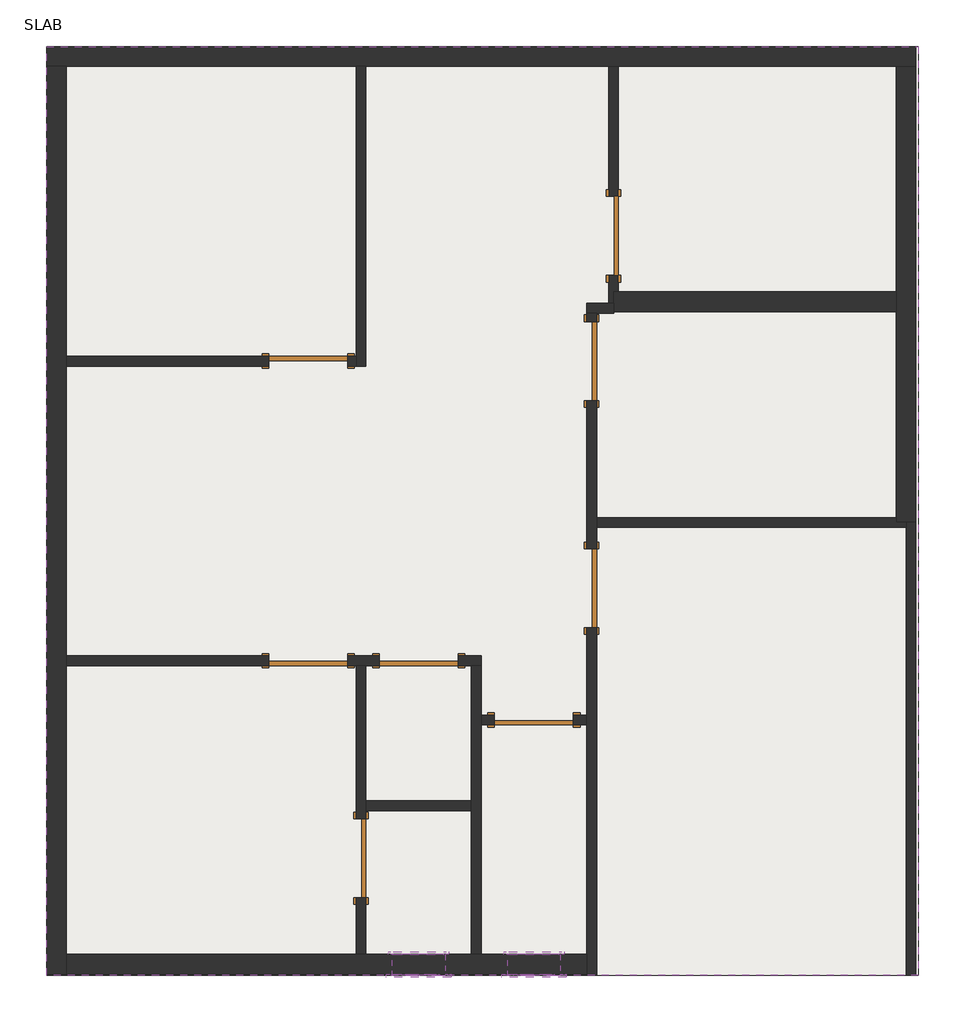
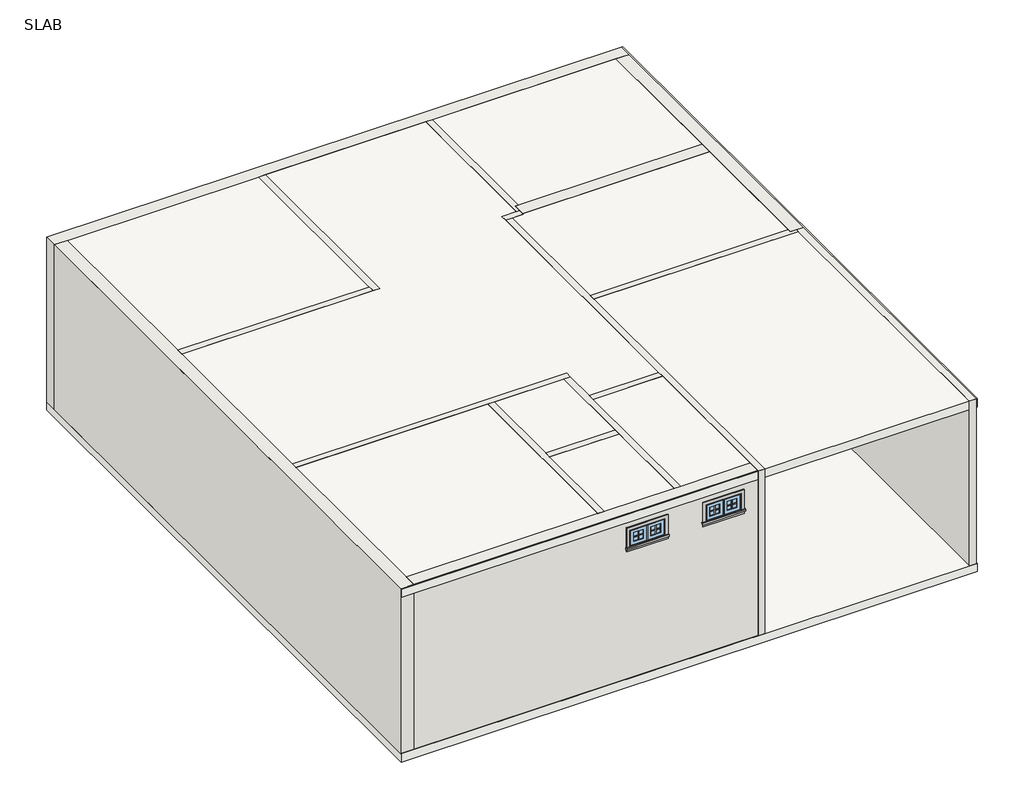
# One storey: 17 walls, 8 doors, 8 proxies, 2 slabs, 2 windows.
"""IFC4 building model written with IfcOpenShell, lengths in millimetres."""

from ifc_helpers import new_model, si_unit, frame, origin, place, context, project, spatial, polyline, outline, extrude, faceted_brep, transform, mapped, element, save
from components import muntin_pattern_2x2_muntin_pattern_2x2_4939cdd6, muntin_pattern_2x2_muntin_pattern_2x2_7edc5815, trim_window_exterior_flat_with_sill_281d40e2, trim_window_interior_flat_picture_frame_d1e4ee8f, door_305aa2a5, door_e5f9f3c4, window_375d1de9

model = new_model("IFC4")

# Units and contexts
model_context = context("Model", 3, world=origin())
ifc_project = project(units=[si_unit("LENGTHUNIT", "METRE", prefix="MILLI")], contexts=[model_context])

# Site, building, storey
site = spatial("IfcSite", under=ifc_project)
building = spatial("IfcBuilding", under=site)
storey = spatial("IfcBuildingStorey", under=building, Name="SLAB", Elevation=3657.6)

# Proxies
placement = place(None, origin())
muntin_pattern_2x2_muntin_pattern_2x2_shape = muntin_pattern_2x2_muntin_pattern_2x2_4939cdd6(model_context)
element("IfcBuildingElementProxy", 1, Name="Muntin Pattern_2x2 : Muntin Pattern_2x2", ObjectType="Muntin Pattern_2x2 : Muntin Pattern_2x2", at=placement, inside=storey, context=model_context, shape_type="MappedRepresentation", body=[
    mapped(muntin_pattern_2x2_muntin_pattern_2x2_shape, transform((-5153.2054063, 91.6138401, 6165.85), x_axis=(-1.0, 0.0, 0.0), y_axis=(0.0, -1.0, 0.0), z_axis=(0.0, 0.0, 1.0))),
])
element("IfcBuildingElementProxy", 2, Name="Muntin Pattern_2x2 : Muntin Pattern_2x2", ObjectType="Muntin Pattern_2x2 : Muntin Pattern_2x2", at=placement, inside=storey, context=model_context, shape_type="MappedRepresentation", body=[
    mapped(muntin_pattern_2x2_muntin_pattern_2x2_shape, transform((-3819.7054063, 91.6138401, 6165.85), x_axis=(-1.0, 0.0, 0.0), y_axis=(0.0, -1.0, 0.0), z_axis=(0.0, 0.0, 1.0))),
])
muntin_pattern_2x2_muntin_pattern_2x2_2_shape = muntin_pattern_2x2_muntin_pattern_2x2_7edc5815(model_context)
element("IfcBuildingElementProxy", 3, Name="Muntin Pattern_2x2 : Muntin Pattern_2x2", ObjectType="Muntin Pattern_2x2 : Muntin Pattern_2x2", at=placement, inside=storey, context=model_context, shape_type="MappedRepresentation", body=[
    mapped(muntin_pattern_2x2_muntin_pattern_2x2_2_shape, transform((-5454.8304063, 91.6138401, 6165.85), x_axis=(1.0, 0.0, 0.0), y_axis=(0.0, 1.0, 0.0), z_axis=(0.0, 0.0, 1.0))),
])
element("IfcBuildingElementProxy", 4, Name="Muntin Pattern_2x2 : Muntin Pattern_2x2", ObjectType="Muntin Pattern_2x2 : Muntin Pattern_2x2", at=placement, inside=storey, context=model_context, shape_type="MappedRepresentation", body=[
    mapped(muntin_pattern_2x2_muntin_pattern_2x2_2_shape, transform((-4121.3304063, 91.6138401, 6165.85), x_axis=(1.0, 0.0, 0.0), y_axis=(0.0, 1.0, 0.0), z_axis=(0.0, 0.0, 1.0))),
])
trim_window_exterior_flat_with_sill_shape = trim_window_exterior_flat_with_sill_281d40e2(model_context)
element("IfcBuildingElementProxy", 5, Name="Trim-Window-Exterior-Flat : with Sill", ObjectType="Trim-Window-Exterior-Flat : with Sill", at=placement, inside=storey, context=model_context, shape_type="MappedRepresentation", body=[
    mapped(trim_window_exterior_flat_with_sill_shape, transform((-5304.0179063, 82.0888401, 6400.8), x_axis=(1.0, 0.0, 0.0), y_axis=(0.0, 0.0, 1.0), z_axis=(0.0, -1.0, 0.0))),
])
element("IfcBuildingElementProxy", 6, Name="Trim-Window-Exterior-Flat : with Sill", ObjectType="Trim-Window-Exterior-Flat : with Sill", at=placement, inside=storey, context=model_context, shape_type="MappedRepresentation", body=[
    mapped(trim_window_exterior_flat_with_sill_shape, transform((-3970.5179063, 82.0888401, 6400.8), x_axis=(1.0, 0.0, 0.0), y_axis=(0.0, 0.0, 1.0), z_axis=(0.0, -1.0, 0.0))),
])
trim_window_interior_flat_picture_frame_shape = trim_window_interior_flat_picture_frame_d1e4ee8f(model_context)
element("IfcBuildingElementProxy", 7, Name="Trim-Window-Interior-Flat : Picture Frame", ObjectType="Trim-Window-Interior-Flat : Picture Frame", at=placement, inside=storey, context=model_context, shape_type="MappedRepresentation", body=[
    mapped(trim_window_interior_flat_picture_frame_shape, transform((-5304.0179063, 310.6888401, 6400.8), x_axis=(-1.0, 0.0, 0.0), y_axis=(0.0, 0.0, 1.0), z_axis=(0.0, 1.0, 0.0))),
])
element("IfcBuildingElementProxy", 8, Name="Trim-Window-Interior-Flat : Picture Frame", ObjectType="Trim-Window-Interior-Flat : Picture Frame", at=placement, inside=storey, context=model_context, shape_type="MappedRepresentation", body=[
    mapped(trim_window_interior_flat_picture_frame_shape, transform((-3970.5179063, 310.6888401, 6400.8), x_axis=(-1.0, 0.0, 0.0), y_axis=(0.0, 0.0, 1.0), z_axis=(0.0, 1.0, 0.0))),
])

# Doors
door_shape = door_305aa2a5(model_context)
element("IfcDoor", 9, ObjectType="Single-Flush : 36\" x 84\"", at=placement, inside=storey, context=model_context, shape_type="MappedRepresentation", body=[
    mapped(door_shape, transform((-5970.7679063, 1421.9388401, 3657.6), x_axis=(0.0, 1.0, 0.0), y_axis=(-1.0, 0.0, 0.0), z_axis=(0.0, 0.0, 1.0))),
])
element("IfcDoor", 10, ObjectType="Single-Flush : 36\" x 84\"", at=placement, inside=storey, context=model_context, shape_type="MappedRepresentation", body=[
    mapped(door_shape, transform((-5304.0179063, 3707.9388401, 3657.6), x_axis=(1.0, 0.0, 0.0), y_axis=(0.0, 1.0, 0.0), z_axis=(0.0, 0.0, 1.0))),
])
element("IfcDoor", 11, ObjectType="Single-Flush : 36\" x 84\"", at=placement, inside=storey, context=model_context, shape_type="MappedRepresentation", body=[
    mapped(door_shape, transform((-6580.3679063, 3707.9388401, 3657.6), x_axis=(1.0, 0.0, 0.0), y_axis=(0.0, 1.0, 0.0), z_axis=(0.0, 0.0, 1.0))),
])
element("IfcDoor", 12, ObjectType="Single-Flush : 36\" x 84\"", at=placement, inside=storey, context=model_context, shape_type="MappedRepresentation", body=[
    mapped(door_shape, transform((-3303.7679063, 7175.0388401, 3657.6), x_axis=(0.0, 1.0, 0.0), y_axis=(-1.0, 0.0, 0.0), z_axis=(0.0, 0.0, 1.0))),
])
door_2_shape = door_e5f9f3c4(model_context)
element("IfcDoor", 13, ObjectType="Single-Flush : 36\" x 84\"", at=placement, inside=storey, context=model_context, shape_type="MappedRepresentation", body=[
    mapped(door_2_shape, transform((-3303.7679063, 4546.1388401, 3657.6), x_axis=(0.0, -1.0, 0.0), y_axis=(1.0, 0.0, 0.0), z_axis=(0.0, 0.0, 1.0))),
])
element("IfcDoor", 14, ObjectType="Single-Flush : 36\" x 84\"", at=placement, inside=storey, context=model_context, shape_type="MappedRepresentation", body=[
    mapped(door_2_shape, transform((-3970.5179063, 3022.1388401, 3657.6), x_axis=(-1.0, 0.0, 0.0), y_axis=(0.0, -1.0, 0.0), z_axis=(0.0, 0.0, 1.0))),
])
element("IfcDoor", 15, ObjectType="Single-Flush : 36\" x 84\"", at=placement, inside=storey, context=model_context, shape_type="MappedRepresentation", body=[
    mapped(door_2_shape, transform((-6580.3679063, 7175.0388401, 3657.6), x_axis=(1.0, 0.0, 0.0), y_axis=(0.0, 1.0, 0.0), z_axis=(0.0, 0.0, 1.0))),
])
element("IfcDoor", 16, ObjectType="Single-Flush : 36\" x 84\"", at=placement, inside=storey, context=model_context, shape_type="MappedRepresentation", body=[
    mapped(door_2_shape, transform((-3049.7679063, 8622.8388401, 3657.6), x_axis=(0.0, -1.0, 0.0), y_axis=(1.0, 0.0, 0.0), z_axis=(0.0, 0.0, 1.0))),
])

# Slabs
element("IfcSlab", 17, ObjectType="SLAB 6\"", at=placement, inside=storey, context=model_context, shape_type="SweptSolid", body=[
    extrude(outline(polyline([(449.0820937, 10813.5888401), (474.4820937, 10813.5888401), (474.4820937, 69.3888401), (-9609.3179063, 69.3888401), (-9609.3179063, 10813.5888401), (449.0820937, 10813.5888401)])), frame((0.0, 0.0, 3505.2), z_axis=(0.0, 0.0, 1.0), x_axis=(1.0, 0.0, 0.0)), (0.0, 0.0, 1.0), 152.4),
])
element("IfcSlab", 18, ObjectType="SLAB 6\"", at=placement, inside=storey, context=model_context, shape_type="SweptSolid", body=[
    extrude(outline(polyline([(449.0820937, 10813.5888401), (474.4820937, 10813.5888401), (474.4820937, 69.3888401), (-9609.3179063, 69.3888401), (-9609.3179063, 10813.5888401), (449.0820937, 10813.5888401)])), frame((0.0, 0.0, 6553.2), z_axis=(0.0, 0.0, 1.0), x_axis=(1.0, 0.0, 0.0)), (0.0, 0.0, 1.0), 152.4),
])

# Walls
element("IfcWall", 19, ObjectType="wall 4.5\"", at=placement, inside=storey, context=model_context, shape_type="Brep", body=[
    faceted_brep([(-3246.6179063, 7632.2388401, 5791.2), (-3246.6179063, 7632.2388401, 3657.6), (-3246.6179063, 7727.4888401, 3657.6), (-3246.6179063, 7727.4888401, 6705.6), (-3246.6179063, 5365.2888401, 6705.6), (-3246.6179063, 5250.9888401, 6705.6), (-3246.6179063, 69.3888401, 6705.6), (-3246.6179063, 69.3888401, 3657.6), (-3246.6179063, 4088.9388401, 3657.6), (-3246.6179063, 4088.9388401, 5791.2), (-3246.6179063, 5003.3388401, 5791.2), (-3246.6179063, 5003.3388401, 3657.6), (-3246.6179063, 5250.9888401, 3657.6), (-3246.6179063, 5365.2888401, 3657.6), (-3246.6179063, 6717.8388401, 3657.6), (-3246.6179063, 6717.8388401, 5791.2), (-3360.9179063, 7727.4888401, 3657.6), (-3360.9179063, 7632.2388401, 3657.6), (-3360.9179063, 7632.2388401, 5791.2), (-3360.9179063, 6717.8388401, 5791.2), (-3360.9179063, 6717.8388401, 3657.6), (-3360.9179063, 5003.3388401, 3657.6), (-3360.9179063, 5003.3388401, 5791.2), (-3360.9179063, 4088.9388401, 5791.2), (-3360.9179063, 4088.9388401, 3657.6), (-3360.9179063, 3079.2888401, 3657.6), (-3360.9179063, 2964.9888401, 3657.6), (-3360.9179063, 69.3888401, 3657.6), (-3360.9179063, 69.3888401, 6705.6), (-3360.9179063, 2964.9888401, 6705.6), (-3360.9179063, 3079.2888401, 6705.6), (-3360.9179063, 7727.4888401, 6705.6)], [[[0, 1, 2, 3, 4, 5, 6, 7, 8, 9, 10, 11, 12, 13, 14, 15]], [[16, 17, 18, 19, 20, 21, 22, 23, 24, 25, 26, 27, 28, 29, 30, 31]], [[27, 26, 25, 24, 8, 7]], [[2, 1, 17, 16]], [[14, 13, 12, 11, 21, 20]], [[6, 5, 4, 3, 31, 30, 29, 28]], [[7, 6, 28, 27]], [[3, 2, 16, 31]], [[9, 8, 24, 23]], [[10, 9, 23, 22]], [[11, 10, 22, 21]], [[18, 17, 1, 0]], [[19, 18, 0, 15]], [[20, 19, 15, 14]]]),
])
element("IfcWall", 20, ObjectType="wall 4.5\"", at=placement, inside=storey, context=model_context, shape_type="Brep", body=[
    faceted_brep([(334.7820937, 5308.1388401, 3657.6), (334.7820937, 5250.9888401, 3657.6), (334.7820937, 69.3888401, 3657.6), (334.7820937, 69.3888401, 6705.6), (334.7820937, 5250.9888401, 6705.6), (334.7820937, 5308.1388401, 6705.6), (449.0820937, 5308.1388401, 3657.6), (449.0820937, 5308.1388401, 6705.6), (449.0820937, 69.3888401, 6705.6), (449.0820937, 69.3888401, 3657.6)], [[[0, 1, 2, 3, 4, 5]], [[6, 7, 8, 9]], [[2, 1, 0, 6, 9]], [[3, 2, 9, 8]], [[5, 4, 3, 8, 7]], [[0, 5, 7, 6]]]),
])
element("IfcWall", 21, ObjectType="wall 4.5\"", at=placement, inside=storey, context=model_context, shape_type="SweptSolid", body=[
    extrude(outline(polyline([(334.7820937, 5250.9888401), (-3246.6179063, 5250.9888401), (-3246.6179063, 5365.2888401), (220.4820937, 5365.2888401), (220.4820937, 5308.1388401), (334.7820937, 5308.1388401), (334.7820937, 5250.9888401)])), frame((0.0, 0.0, 3657.6), z_axis=(0.0, 0.0, 1.0), x_axis=(1.0, 0.0, 0.0)), (0.0, 0.0, 1.0), 3048.0),
])
element("IfcWall", 22, ObjectType="wall 4.5\"", at=placement, inside=storey, context=model_context, shape_type="Brep", body=[
    faceted_brep([(-3106.9179063, 8165.6388401, 5791.2), (-3106.9179063, 8165.6388401, 3657.6), (-3106.9179063, 7841.7888401, 3657.6), (-3106.9179063, 7841.7888401, 6705.6), (-3106.9179063, 10584.9888401, 6705.6), (-3106.9179063, 10584.9888401, 3657.6), (-3106.9179063, 9080.0388401, 3657.6), (-3106.9179063, 9080.0388401, 5791.2), (-2992.6179063, 7975.1388401, 3657.6), (-2992.6179063, 8165.6388401, 3657.6), (-2992.6179063, 8165.6388401, 5791.2), (-2992.6179063, 9080.0388401, 5791.2), (-2992.6179063, 9080.0388401, 3657.6), (-2992.6179063, 10584.9888401, 3657.6), (-2992.6179063, 10584.9888401, 6705.6), (-2992.6179063, 7975.1388401, 6705.6), (-3049.7679063, 7975.1388401, 3657.6), (-3049.7679063, 7841.7888401, 3657.6), (-3049.7679063, 7841.7888401, 6705.6), (-3049.7679063, 7975.1388401, 6705.6)], [[[0, 1, 2, 3, 4, 5, 6, 7]], [[8, 9, 10, 11, 12, 13, 14, 15]], [[6, 5, 13, 12]], [[2, 1, 9, 8, 16, 17]], [[4, 3, 18, 19, 15, 14]], [[5, 4, 14, 13]], [[3, 2, 17, 18]], [[17, 16, 19, 18]], [[16, 8, 15, 19]], [[10, 9, 1, 0]], [[11, 10, 0, 7]], [[12, 11, 7, 6]]]),
])
element("IfcWall", 23, ObjectType="wall 4.5\"", at=placement, inside=storey, context=model_context, shape_type="Brep", body=[
    faceted_brep([(-6027.9179063, 10584.9888401, 3657.6), (-6027.9179063, 7232.1888401, 3657.6), (-6027.9179063, 7117.8888401, 3657.6), (-6027.9179063, 7117.8888401, 6705.6), (-6027.9179063, 7232.1888401, 6705.6), (-6027.9179063, 10584.9888401, 6705.6), (-5913.6179063, 10584.9888401, 3657.6), (-5913.6179063, 10584.9888401, 6705.6), (-5913.6179063, 7117.8888401, 6705.6), (-5913.6179063, 7117.8888401, 3657.6)], [[[0, 1, 2, 3, 4, 5]], [[6, 7, 8, 9]], [[2, 1, 0, 6, 9]], [[5, 4, 3, 8, 7]], [[0, 5, 7, 6]], [[3, 2, 9, 8]]]),
])
element("IfcWall", 24, ObjectType="wall 4.5\"", at=placement, inside=storey, context=model_context, shape_type="SweptSolid", body=[
    extrude(outline(polyline([(5791.2, -6123.1679063), (3657.6, -6123.1679063), (3657.6, -6027.9179063), (6705.6, -6027.9179063), (6705.6, -9380.7179063), (3657.6, -9380.7179063), (3657.6, -7037.5679063), (5791.2, -7037.5679063), (5791.2, -6123.1679063)])), frame((0.0, 7117.8888401, 0.0), z_axis=(0.0, 1.0, 0.0), x_axis=(0.0, 0.0, 1.0)), (0.0, 0.0, 1.0), 114.3),
])
element("IfcWall", 25, ObjectType="wall 4.5\"", at=placement, inside=storey, context=model_context, shape_type="Brep", body=[
    faceted_brep([(-6123.1679063, 3650.7888401, 5791.2), (-6123.1679063, 3650.7888401, 3657.6), (-6027.9179063, 3650.7888401, 3657.6), (-5913.6179063, 3650.7888401, 3657.6), (-5761.2179063, 3650.7888401, 3657.6), (-5761.2179063, 3650.7888401, 5791.2), (-4846.8179063, 3650.7888401, 5791.2), (-4846.8179063, 3650.7888401, 3657.6), (-4694.4179063, 3650.7888401, 3657.6), (-4580.1179063, 3650.7888401, 3657.6), (-4580.1179063, 3650.7888401, 6705.6), (-4694.4179063, 3650.7888401, 6705.6), (-5913.6179063, 3650.7888401, 6705.6), (-6027.9179063, 3650.7888401, 6705.6), (-9380.7179063, 3650.7888401, 6705.6), (-9380.7179063, 3650.7888401, 3657.6), (-7037.5679063, 3650.7888401, 3657.6), (-7037.5679063, 3650.7888401, 5791.2), (-5761.2179063, 3765.0888401, 3657.6), (-6123.1679063, 3765.0888401, 3657.6), (-6123.1679063, 3765.0888401, 5791.2), (-7037.5679063, 3765.0888401, 5791.2), (-7037.5679063, 3765.0888401, 3657.6), (-9380.7179063, 3765.0888401, 3657.6), (-9380.7179063, 3765.0888401, 6705.6), (-4580.1179063, 3765.0888401, 6705.6), (-4580.1179063, 3765.0888401, 3657.6), (-4846.8179063, 3765.0888401, 3657.6), (-4846.8179063, 3765.0888401, 5791.2), (-5761.2179063, 3765.0888401, 5791.2)], [[[0, 1, 2, 3, 4, 5, 6, 7, 8, 9, 10, 11, 12, 13, 14, 15, 16, 17]], [[18, 19, 20, 21, 22, 23, 24, 25, 26, 27, 28, 29]], [[9, 8, 7, 27, 26]], [[16, 15, 23, 22]], [[4, 3, 2, 1, 19, 18]], [[14, 13, 12, 11, 10, 25, 24]], [[15, 14, 24, 23]], [[10, 9, 26, 25]], [[28, 27, 7, 6]], [[29, 28, 6, 5]], [[18, 29, 5, 4]], [[20, 19, 1, 0]], [[21, 20, 0, 17]], [[22, 21, 17, 16]]]),
])
element("IfcWall", 26, ObjectType="wall 4.5\"", at=placement, inside=storey, context=model_context, shape_type="Brep", body=[
    faceted_brep([(-4694.4179063, 3650.7888401, 3657.6), (-4694.4179063, 2088.6888401, 3657.6), (-4694.4179063, 1974.3888401, 3657.6), (-4694.4179063, 310.6888401, 3657.6), (-4694.4179063, 310.6888401, 6705.6), (-4694.4179063, 1974.3888401, 6705.6), (-4694.4179063, 2088.6888401, 6705.6), (-4694.4179063, 3650.7888401, 6705.6), (-4580.1179063, 3650.7888401, 3657.6), (-4580.1179063, 3650.7888401, 6705.6), (-4580.1179063, 3079.2888401, 6705.6), (-4580.1179063, 2964.9888401, 6705.6), (-4580.1179063, 310.6888401, 6705.6), (-4580.1179063, 310.6888401, 3657.6), (-4580.1179063, 2964.9888401, 3657.6), (-4580.1179063, 3079.2888401, 3657.6)], [[[0, 1, 2, 3, 4, 5, 6, 7]], [[8, 9, 10, 11, 12, 13, 14, 15]], [[3, 2, 1, 0, 8, 15, 14, 13]], [[7, 6, 5, 4, 12, 11, 10, 9]], [[0, 7, 9, 8]], [[4, 3, 13, 12]]]),
])
element("IfcWall", 27, ObjectType="wall 4.5\"", at=placement, inside=storey, context=model_context, shape_type="Brep", body=[
    faceted_brep([(-5913.6179063, 1879.1388401, 5791.2), (-5913.6179063, 1879.1388401, 3657.6), (-5913.6179063, 1974.3888401, 3657.6), (-5913.6179063, 2088.6888401, 3657.6), (-5913.6179063, 3650.7888401, 3657.6), (-5913.6179063, 3650.7888401, 6705.6), (-5913.6179063, 2088.6888401, 6705.6), (-5913.6179063, 1974.3888401, 6705.6), (-5913.6179063, 310.6888401, 6705.6), (-5913.6179063, 310.6888401, 3657.6), (-5913.6179063, 964.7388401, 3657.6), (-5913.6179063, 964.7388401, 5791.2), (-6027.9179063, 3650.7888401, 3657.6), (-6027.9179063, 1879.1388401, 3657.6), (-6027.9179063, 1879.1388401, 5791.2), (-6027.9179063, 964.7388401, 5791.2), (-6027.9179063, 964.7388401, 3657.6), (-6027.9179063, 310.6888401, 3657.6), (-6027.9179063, 310.6888401, 6705.6), (-6027.9179063, 3650.7888401, 6705.6)], [[[0, 1, 2, 3, 4, 5, 6, 7, 8, 9, 10, 11]], [[12, 13, 14, 15, 16, 17, 18, 19]], [[10, 9, 17, 16]], [[4, 3, 2, 1, 13, 12]], [[8, 7, 6, 5, 19, 18]], [[9, 8, 18, 17]], [[5, 4, 12, 19]], [[14, 13, 1, 0]], [[15, 14, 0, 11]], [[16, 15, 11, 10]]]),
])
element("IfcWall", 28, ObjectType="wall 4.5\"", at=placement, inside=storey, context=model_context, shape_type="SweptSolid", body=[
    extrude(outline(polyline([(-5913.6179063, 2088.6888401), (-4694.4179063, 2088.6888401), (-4694.4179063, 1974.3888401), (-5913.6179063, 1974.3888401), (-5913.6179063, 2088.6888401)])), frame((0.0, 0.0, 3657.6), z_axis=(0.0, 0.0, 1.0), x_axis=(1.0, 0.0, 0.0)), (0.0, 0.0, 1.0), 3048.0),
])
element("IfcWall", 29, ObjectType="wall 4.5\"", at=placement, inside=storey, context=model_context, shape_type="SweptSolid", body=[
    extrude(outline(polyline([(3657.6, -4580.1179063), (3657.6, -4427.7179063), (5791.2, -4427.7179063), (5791.2, -3513.3179063), (3657.6, -3513.3179063), (3657.6, -3360.9179063), (6705.6, -3360.9179063), (6705.6, -4580.1179063), (3657.6, -4580.1179063)])), frame((0.0, 2964.9888401, 0.0), z_axis=(0.0, 1.0, 0.0), x_axis=(0.0, 0.0, 1.0)), (0.0, 0.0, 1.0), 114.3),
])
element("IfcWall", 30, ObjectType="wall 4.5\"", at=placement, inside=storey, context=model_context, shape_type="Brep", body=[
    faceted_brep([(-3360.9179063, 7727.4888401, 3657.6), (-3246.6179063, 7727.4888401, 3657.6), (-3049.7679063, 7727.4888401, 3657.6), (-3049.7679063, 7727.4888401, 6705.6), (-3246.6179063, 7727.4888401, 6705.6), (-3360.9179063, 7727.4888401, 6705.6), (-3360.9179063, 7841.7888401, 3657.6), (-3360.9179063, 7841.7888401, 6705.6), (-3106.9179063, 7841.7888401, 6705.6), (-3049.7679063, 7841.7888401, 6705.6), (-3049.7679063, 7841.7888401, 3657.6), (-3106.9179063, 7841.7888401, 3657.6), (-3049.7679063, 7746.5388401, 3657.6), (-3049.7679063, 7746.5388401, 6705.6)], [[[0, 1, 2, 3, 4, 5]], [[6, 7, 8, 9, 10, 11]], [[2, 1, 0, 6, 11, 10, 12]], [[3, 2, 12, 10, 9, 13]], [[5, 4, 3, 13, 9, 8, 7]], [[0, 5, 7, 6]]]),
])
element("IfcWall", 31, ObjectType="wall 9\"", at=placement, inside=storey, context=model_context, shape_type="Brep", body=[
    faceted_brep([(-9609.3179063, 10584.9888401, 3657.6), (-9380.7179063, 10584.9888401, 3657.6), (-6027.9179063, 10584.9888401, 3657.6), (-5913.6179063, 10584.9888401, 3657.6), (-3106.9179063, 10584.9888401, 3657.6), (-2992.6179063, 10584.9888401, 3657.6), (220.4820937, 10584.9888401, 3657.6), (449.0820937, 10584.9888401, 3657.6), (449.0820937, 10584.9888401, 6705.6), (220.4820937, 10584.9888401, 6705.6), (-2992.6179063, 10584.9888401, 6705.6), (-3106.9179063, 10584.9888401, 6705.6), (-5913.6179063, 10584.9888401, 6705.6), (-6027.9179063, 10584.9888401, 6705.6), (-9380.7179063, 10584.9888401, 6705.6), (-9609.3179063, 10584.9888401, 6705.6), (-9609.3179063, 10813.5888401, 3657.6), (-9609.3179063, 10813.5888401, 6705.6), (449.0820937, 10813.5888401, 6705.6), (449.0820937, 10813.5888401, 3657.6)], [[[0, 1, 2, 3, 4, 5, 6, 7, 8, 9, 10, 11, 12, 13, 14, 15]], [[16, 17, 18, 19]], [[7, 6, 5, 4, 3, 2, 1, 0, 16, 19]], [[15, 14, 13, 12, 11, 10, 9, 8, 18, 17]], [[8, 7, 19, 18]], [[0, 15, 17, 16]]]),
])
element("IfcWall", 32, ObjectType="wall 9\"", at=placement, inside=storey, context=model_context, shape_type="Brep", body=[
    faceted_brep([(220.4820937, 10584.9888401, 3657.6), (220.4820937, 7975.1388401, 3657.6), (220.4820937, 7746.5388401, 3657.6), (220.4820937, 5365.2888401, 3657.6), (220.4820937, 5308.1388401, 3657.6), (220.4820937, 5308.1388401, 6705.6), (220.4820937, 5365.2888401, 6705.6), (220.4820937, 7746.5388401, 6705.6), (220.4820937, 7975.1388401, 6705.6), (220.4820937, 10584.9888401, 6705.6), (449.0820937, 10584.9888401, 3657.6), (449.0820937, 10584.9888401, 6705.6), (449.0820937, 5308.1388401, 6705.6), (449.0820937, 5308.1388401, 3657.6), (334.7820937, 5308.1388401, 3657.6), (334.7820937, 5308.1388401, 6705.6)], [[[0, 1, 2, 3, 4, 5, 6, 7, 8, 9]], [[10, 11, 12, 13]], [[4, 3, 2, 1, 0, 10, 13, 14]], [[5, 4, 14, 13, 12, 15]], [[9, 8, 7, 6, 5, 15, 12, 11]], [[0, 9, 11, 10]]]),
])
element("IfcWall", 33, ObjectType="wall 9\"", at=placement, inside=storey, context=model_context, shape_type="Brep", body=[
    faceted_brep([(-9609.3179063, 10584.9888401, 3657.6), (-9609.3179063, 82.0888401, 3657.6), (-9609.3179063, 82.0888401, 6705.6), (-9609.3179063, 10584.9888401, 6705.6), (-9380.7179063, 10584.9888401, 3657.6), (-9380.7179063, 10584.9888401, 6705.6), (-9380.7179063, 7232.1888401, 6705.6), (-9380.7179063, 7117.8888401, 6705.6), (-9380.7179063, 3765.0888401, 6705.6), (-9380.7179063, 3650.7888401, 6705.6), (-9380.7179063, 310.6888401, 6705.6), (-9380.7179063, 82.0888401, 6705.6), (-9380.7179063, 82.0888401, 3657.6), (-9380.7179063, 310.6888401, 3657.6), (-9380.7179063, 3650.7888401, 3657.6), (-9380.7179063, 3765.0888401, 3657.6), (-9380.7179063, 7117.8888401, 3657.6), (-9380.7179063, 7232.1888401, 3657.6)], [[[0, 1, 2, 3]], [[4, 5, 6, 7, 8, 9, 10, 11, 12, 13, 14, 15, 16, 17]], [[1, 0, 4, 17, 16, 15, 14, 13, 12]], [[3, 2, 11, 10, 9, 8, 7, 6, 5]], [[0, 3, 5, 4]], [[2, 1, 12, 11]]]),
])
element("IfcWall", 34, ObjectType="wall 9\"", at=placement, inside=storey, context=model_context, shape_type="Brep", body=[
    faceted_brep([(-9380.7179063, 82.0888401, 3657.6), (-3360.9179063, 82.0888401, 3657.6), (-3360.9179063, 82.0888401, 6705.6), (-9380.7179063, 82.0888401, 6705.6), (-5608.8179063, 82.0888401, 6400.8), (-4999.2179063, 82.0888401, 6400.8), (-4999.2179063, 82.0888401, 6096.0), (-5608.8179063, 82.0888401, 6096.0), (-4275.3179063, 82.0888401, 6400.8), (-3665.7179063, 82.0888401, 6400.8), (-3665.7179063, 82.0888401, 6096.0), (-4275.3179063, 82.0888401, 6096.0), (-9380.7179063, 310.6888401, 3657.6), (-9380.7179063, 310.6888401, 6705.6), (-6027.9179063, 310.6888401, 6705.6), (-5913.6179063, 310.6888401, 6705.6), (-4694.4179063, 310.6888401, 6705.6), (-4580.1179063, 310.6888401, 6705.6), (-3360.9179063, 310.6888401, 6705.6), (-3360.9179063, 310.6888401, 3657.6), (-4580.1179063, 310.6888401, 3657.6), (-4694.4179063, 310.6888401, 3657.6), (-5913.6179063, 310.6888401, 3657.6), (-6027.9179063, 310.6888401, 3657.6), (-5608.8179063, 310.6888401, 6400.8), (-5608.8179063, 310.6888401, 6096.0), (-4999.2179063, 310.6888401, 6096.0), (-4999.2179063, 310.6888401, 6400.8), (-4275.3179063, 310.6888401, 6400.8), (-4275.3179063, 310.6888401, 6096.0), (-3665.7179063, 310.6888401, 6096.0), (-3665.7179063, 310.6888401, 6400.8)], [[[0, 1, 2, 3], [4, 5, 6, 7], [8, 9, 10, 11]], [[12, 13, 14, 15, 16, 17, 18, 19, 20, 21, 22, 23], [24, 25, 26, 27], [28, 29, 30, 31]], [[1, 0, 12, 23, 22, 21, 20, 19]], [[2, 1, 19, 18]], [[3, 2, 18, 17, 16, 15, 14, 13]], [[0, 3, 13, 12]], [[25, 24, 4, 7]], [[26, 25, 7, 6]], [[27, 26, 6, 5]], [[24, 27, 5, 4]], [[29, 28, 8, 11]], [[30, 29, 11, 10]], [[31, 30, 10, 9]], [[28, 31, 9, 8]]]),
])
element("IfcWall", 35, ObjectType="wall 9\"", at=placement, inside=storey, context=model_context, shape_type="Brep", body=[
    faceted_brep([(220.4820937, 7975.1388401, 3657.6), (-2992.6179063, 7975.1388401, 3657.6), (-3049.7679063, 7975.1388401, 3657.6), (-3049.7679063, 7975.1388401, 6705.6), (-2992.6179063, 7975.1388401, 6705.6), (220.4820937, 7975.1388401, 6705.6), (220.4820937, 7746.5388401, 3657.6), (220.4820937, 7746.5388401, 6705.6), (-3049.7679063, 7746.5388401, 6705.6), (-3049.7679063, 7746.5388401, 3657.6), (-3049.7679063, 7841.7888401, 3657.6), (-3049.7679063, 7841.7888401, 6705.6)], [[[0, 1, 2, 3, 4, 5]], [[6, 7, 8, 9]], [[2, 1, 0, 6, 9, 10]], [[3, 2, 10, 9, 8, 11]], [[5, 4, 3, 11, 8, 7]], [[0, 5, 7, 6]]]),
])

# Windows
window_shape = window_375d1de9(model_context)
element("IfcWindow", 36, ObjectType="Window-Casement-Double : 24\"X1'", at=placement, inside=storey, context=model_context, shape_type="MappedRepresentation", body=[
    mapped(window_shape, transform((-5304.0179063, 196.3888401, 5181.6), x_axis=(-1.0, 0.0, 0.0), y_axis=(0.0, -1.0, 0.0), z_axis=(0.0, 0.0, 1.0))),
])
element("IfcWindow", 37, ObjectType="Window-Casement-Double : 24\"X1'", at=placement, inside=storey, context=model_context, shape_type="MappedRepresentation", body=[
    mapped(window_shape, transform((-3970.5179063, 196.3888401, 5181.6), x_axis=(-1.0, 0.0, 0.0), y_axis=(0.0, -1.0, 0.0), z_axis=(0.0, 0.0, 1.0))),
])

save(model, "model.ifc")

# Revit data of these elements
# Type "Muntin Pattern_2x2 : Muntin Pattern_2x2"
#   Width [instance default] = 4' - 0"
#   Thickness = 0' - 0 1/2"
#   Height [instance default] = 4' - 0"
#   Distance = 0' - 0 3/4"
#   Interior Material [instance default] = none
#   Exterior Material [instance default] = none
#   Default Elevation = 0
# Type "Trim-Window-Exterior-Flat : with Sill"
#   Trim Width = 0' - 2 1/4"
#   Trim Thickness_Picture Frame = 0' - 1 1/4"
#   Trim Thickness_with Sill = 0' - 0 3/4"
#   Sill Thickness = 0' - 1 1/4"
#   Opening Width [instance default] = 2' - 0"
#   Opening Height [instance default] = 3' - 0"
#   Default Elevation = 4' - 0"
#   Sill = yes
#   Picture Frame = no
#   Trim Material [instance default] = none
# Type "Trim-Window-Interior-Flat : Picture Frame"
#   Trim Thickness_Picture Frame = 0' - 1 1/4"
#   Trim Width = 0' - 2 1/4"
#   Trim Thickness_with Sill = 0' - 0 3/4"
#   Sill Thickness = 0' - 1 1/4"
#   Opening Width [instance default] = 2' - 0"
#   Opening Height [instance default] = 3' - 0"
#   Default Elevation = 4' - 0"
#   Sill = no
#   Picture Frame = yes
#   Trim Material [instance default] = none
# Type "Single-Flush : 36\" x 84\""
#   Type Mark = "1"
#   Construction Type Id = "MDOOR"
#   Assembly Code = "C1020"
#   Analytic Construction = "Metal"
#   Thickness = 0' - 2"
#   Heat Transfer Coefficient (U) = 0.651978 BTU/(h·ft²·°F)
#   Height = 7' - 0"
#   Trim Projection Ext = 0' - 1"
#   Trim Projection Int = 0' - 1"
#   Trim Width = 0' - 3"
#   Width = 3' - 0"
#   Define Thermal Properties by = 1
#   Define Thermal Properties by = 1
#   Door Material = Door - Panel
#   Frame Material = Door - Frame
#   Visual Light Transmittance = 0
#   Solar Heat Gain Coefficient = 0
#   Function = (empty or 0)
#   Wall Closure = (empty or 0)
# Type "SLAB 6\""
#   Assembly Code = "B1010"
#   Function = 0
#   Layers, outside or top first: 0' - 6" no material (function 1)
# Type "wall 4.5\""
#   Assembly Code = "B2010"
#   Layers, outside or top first: 0' - 4 1/2" no material (function 1)
# Type "wall 9\""
#   Assembly Code = "B2010"
#   Layers, outside or top first: 0' - 9" no material (function 1)
# Type "Window-Casement-Double : 24\"X1'"
#   Type Mark = "V"
#   Fire Rating = "0.5h"
#   Assembly Code = "B2020100"
#   Analytic Construction = "Double glazing - domestic"
#   Frame Extension [instance default] = 0' - 0 1/4"
#   Window Inset [instance default] = 0' - 0"
#   Wall Thickness [instance default] = 0' - 6"
#   Interior Wall Closure [instance default] = 0' - 2 1/4"
#   Half Width = 1' - 0"
#   Visual Light Transmittance = 0.81
#   Thermal Resistance (R) = 1.8146 (h·ft²·°F)/BTU
#   Solar Heat Gain Coefficient = 0.76
#   Rough Width = 2' - 0 1/2"
#   Rough Height = 1' - 0 1/2"
#   Height = 1' - 0"
#   Heat Transfer Coefficient (U) = 0.5511 BTU/(h·ft²·°F)
#   Exterior Wall Closure [instance default] = 0' - 1 1/4"
#   Extension Jamb [instance default] = 0' - 2 1/4"
#   Default Sill Height = 3' - 0"
#   Width = 2' - 0"
#   Muntin Visibility = yes
#   Interior Trim Visibility [instance default] = yes
#   Exterior Trim Visibility [instance default] = yes
#   Extension Jamb Visibility [instance default] = yes
#   Interior Trim Material = Wood - Stained
#   Muntin Pattern = Muntin Pattern_2x2 : Muntin Pattern_2x2
#   Interior Trim = Trim-Window-Interior-Flat : Picture Frame
#   Interior Frame Material = Wood - Stained
#   Glass Panel Material = Glass
#   Exterior Trim Material = Clad - White
#   Exterior Trim = Trim-Window-Exterior-Flat : with Sill
#   Exterior Frame Material = Clad - White
#   Wall Closure = (empty or 0)
# Elements 1, 2, 3, 4 (IfcBuildingElementProxy, "Muntin Pattern_2x2 : Muntin Pattern_2x2")
#   Width = 0' - 6 5/8"
#   Height = 0' - 6 1/2"
#   Interior Material = Wood - Stained
#   Exterior Material = Clad - White
#   Phase Created = New Construction
#   Materials on its faces: "Clad - White", "Wood - Stained"
# Elements 5, 6 (IfcBuildingElementProxy, "Trim-Window-Exterior-Flat : with Sill")
#   Opening Width = 2' - 0"
#   Opening Height = 1' - 0"
#   Trim Material = Clad - White
#   Phase Created = New Construction
#   Materials on its faces: "Clad - White"
# Elements 7, 8 (IfcBuildingElementProxy, "Trim-Window-Interior-Flat : Picture Frame")
#   Opening Width = 2' - 0"
#   Opening Height = 1' - 0"
#   Trim Material = Wood - Stained
#   Phase Created = New Construction
#   Materials on its faces: "Wood - Stained"
# Elements 9, 10, 11, 12, 13, 14, 15, 16 (IfcDoor, "Single-Flush : 36\" x 84\"")
#   Phase Created = New Construction
#   Materials on its faces: "Door - Frame", "Door - Panel"
# Element 17 (IfcSlab, "SLAB 6\"")
#   Height Offset From Level = 0' - 0"
#   Phase Created = New Construction
#   Materials on its faces: "Default Floor"
# Element 18 (IfcSlab, "SLAB 6\"")
#   Height Offset From Level = 10' - 0"
#   Phase Created = New Construction
#   Materials on its faces: "Default Floor"
# Elements 19, 20, 21, 22, 23, 24, 25, 26, 27, 28, 29, 30 (IfcWall, "wall 4.5\"")
#   Top Offset = 0' - 0"
#   Base Offset = 0' - 0"
#   Unconnected Height = 10' - 0"
#   wall height = 10' - 0"
#   Phase Created = New Construction
#   Base Constraint = SLAB
#   Materials on its faces: "Default Wall"
# Elements 31, 32, 33, 34, 35 (IfcWall, "wall 9\"")
#   Top Offset = 0' - 0"
#   Base Offset = 0' - 0"
#   Unconnected Height = 10' - 0"
#   wall height = 10' - 0"
#   Phase Created = New Construction
#   Base Constraint = SLAB
#   Materials on its faces: "Default Wall"
# Element 36 (IfcWindow, "Window-Casement-Double : 24\"X1'")
#   Mark = "9"
#   Window Inset = 0' - 0"
#   Interior Wall Closure = 0' - 2 1/4"
#   Frame Extension = 0' - 0 1/4"
#   Exterior Wall Closure = 0' - 1 1/4"
#   Interior Trim Visibility = yes
#   Exterior Trim Visibility = yes
#   Phase Created = New Construction
#   Materials on its faces: "Wood - Stained", "Glass", "Clad - White"
# Element 37 (IfcWindow, "Window-Casement-Double : 24\"X1'")
#   Mark = "10"
#   Window Inset = 0' - 0"
#   Interior Wall Closure = 0' - 2 1/4"
#   Frame Extension = 0' - 0 1/4"
#   Exterior Wall Closure = 0' - 1 1/4"
#   Interior Trim Visibility = yes
#   Exterior Trim Visibility = yes
#   Phase Created = New Construction
#   Materials on its faces: "Wood - Stained", "Glass", "Clad - White"
# Materials
#   "Door - Panel": class "Wood", colour RGB 210 159 95, transparency 0, Cost = 0
#   "Door - Frame": colour RGB 118 70 51, transparency 0, Cost = 0
#   "Wood - Stained": class "Wood", colour RGB 224 178 126, transparency 0, Cost = 0
#   "Glass": class "Glass", colour RGB 0 128 192, transparency 0.75, Description = "Soda Lime Glass", Cost = 0
#   "Clad - White": class "Wood", colour RGB 242 242 238, transparency 0, Cost = 0
#   "Default Floor": colour RGB 128 128 128, transparency 0, Cost = 0
#   "Default Wall": colour RGB 128 128 128, transparency 0, Cost = 0
